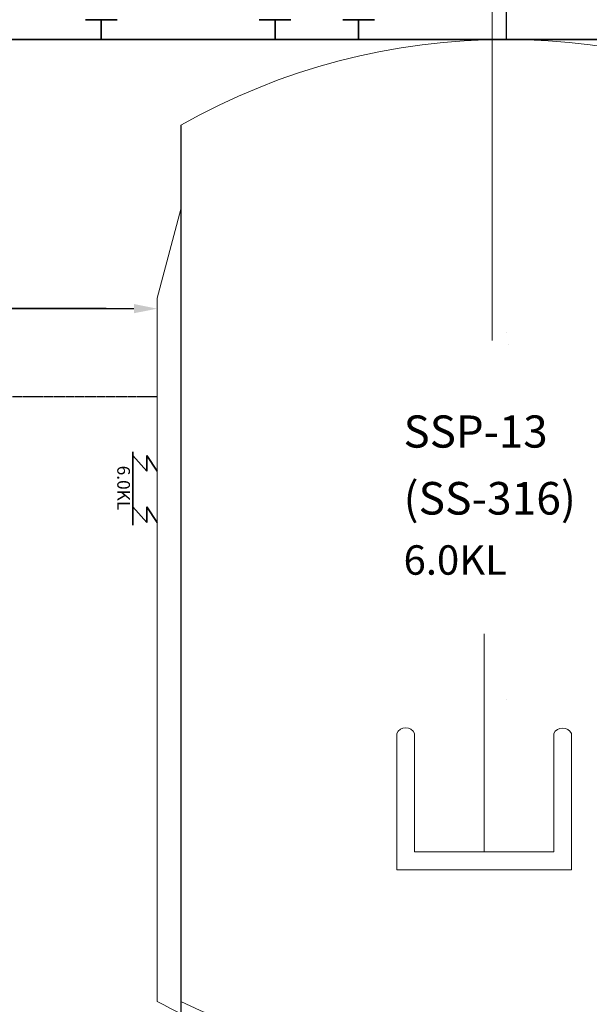
# Model space of a CAD drawing. Units: millimetres. Extents: x 353872 to 441597, y 126154 to 187356.
# Tile 8 of 28: x 390443 to 394852, y 141663 to 149281. Entities that reach past the tile are written whole.
import ezdxf

# ---------------------------------------------------------------- set-up
doc = ezdxf.new("R2010")
doc.units = ezdxf.units.MM
doc.linetypes.add('ACAD_ISO02W100', pattern=[15, 12, -3])
for name, color, linetype, lineweight in [('A-ANNO-DIMS', 2, 'Continuous', 18), ('P-ANNO-SYMB', 7, 'Continuous', 18), ('P-ANNO-TEXT', 7, 'Continuous', 25), ('P-BNDY', 4, 'ACAD_ISO02W100', 25), ('P-INST-SIGN', 4, 'Continuous', 18), ('P-PIPE', 3, 'Continuous', 35), ('P-PIPE-FITT', 6, 'Continuous', 25)]:
    doc.layers.add(name, color=color, linetype=linetype, lineweight=lineweight)
doc.layers.add('AC-UINT', color=2, linetype='Continuous')
doc.styles.get("Standard").update_dxf_attribs({"font": 'arial.ttf'})
doc.dimstyles.get("Standard").update_dxf_attribs({"dimtxt": 0.18, "dimasz": 0.18, "dimexe": 0.18, "dimexo": 0.0625, "dimgap": 0.09, "dimtad": 0, "dimtih": 1, "dimtoh": 1, "dimdec": 4, "dimzin": 0, "dimdsep": 46, "dimtxsty": 'Standard', "dimcen": 0.09, "dimadec": 0, "dimazin": 0, "dimtfac": 1, "dimtdec": 4, "dimtofl": 0, "dimtmove": 0, "dimatfit": 3, "dimfxl": 1, "dimtolj": 1, "dimtzin": 0, "dimarcsym": 0})

# ---------------------------------------------------------------- blocks, each defined once
blk = doc.blocks.new('DFSG')
at = {"layer": 'AC-UINT', "ltscale": 3}
blk.add_line((94.3237, -27.1601), (94.091, -27.1601), dxfattribs=at)
blk.add_solid([(94.091, -27.1214), (94.0909, -27.1989), (93.8965, -27.1598)], dxfattribs=at)
blk = doc.blocks.new('*D29')
at = {"layer": 'A-ANNO-DIMS', "color": 0, "lineweight": -2, "transparency": 16777216}
for p, q in [((391689.9, 148464.5), (391689.9, 133812.7)), ((396727.5, 148464.5), (396727.5, 133812.7)), ((391690.1, 133812.8), (394208.4, 133812.8)), ((396727.3, 133812.8), (394209.1, 133812.8))]:
    blk.add_line(p, q, dxfattribs=at)
at = {"layer": 'A-ANNO-DIMS', "color": 0, "transparency": 16777216}
for points in [[(391690.1, 133812.9), (391690.1, 133812.8), (391689.9, 133812.8)], [(396727.3, 133812.9), (396727.3, 133812.8), (396727.5, 133812.8)]]:
    blk.add_solid(points, dxfattribs=at)
at = {"layer": 'Defpoints', "color": 0, "transparency": 16777216}
for p in [(391689.9, 148464.5), (396727.5, 148464.5), (396727.5, 133812.8)]:
    blk.add_point(p, dxfattribs=at)
at = {"layer": 'A-ANNO-DIMS', "color": 0, "transparency": 16777216, "insert": (394208.7, 133812.8), "char_height": 0.18, "attachment_point": 5}
blk.add_mtext('\\A1;5038', dxfattribs=at)
blk = doc.blocks.new('*D35')
at = {"layer": 'A-ANNO-DIMS', "color": 0, "lineweight": -2, "transparency": 16777216}
for p, q in [((394208.5, 152192.2), (394208.7, 152192.2)), ((394208.7, 152192.2), (394208.7, 149129.3)), ((394208.6, 144024.1), (394208.8, 144024.1)), ((394208.7, 144024), (394208.7, 144024.2))]:
    blk.add_line(p, q, dxfattribs=at)
at = {"layer": 'A-ANNO-DIMS', "color": 0, "transparency": 16777216}
blk.add_solid([(394208.7, 149129.3), (394208.7, 149129.3), (394208.7, 149129.2)], dxfattribs=at)
at = {"layer": 'Defpoints', "color": 0, "transparency": 16777216}
for p in [(394208.7, 149129.2), (394208.7, 144024.1)]:
    blk.add_point(p, dxfattribs=at)
at = {"layer": 'A-ANNO-DIMS', "color": 0, "transparency": 16777216, "insert": (394208.1, 152192.2), "char_height": 0.18, "attachment_point": 5}
blk.add_mtext('\\A1;R5105', dxfattribs=at)
blk = doc.blocks.new('*D36')
at = {"layer": 'A-ANNO-DIMS', "color": 0, "lineweight": -2, "transparency": 16777216}
for p, q in [((394208.6, 146860.2), (394208.8, 146860.2)), ((394208.7, 146860.2), (394208.7, 146860.3)), ((394208.7, 137652.4), (394208.7, 141105.1)), ((394208.5, 137652.4), (394208.7, 137652.4))]:
    blk.add_line(p, q, dxfattribs=at)
at = {"layer": 'A-ANNO-DIMS', "color": 0, "transparency": 16777216}
blk.add_solid([(394208.7, 141105.1), (394208.7, 141105.1), (394208.7, 141105.3)], dxfattribs=at)
at = {"layer": 'Defpoints', "color": 0, "transparency": 16777216}
for p in [(394208.7, 146860.2), (394208.7, 141105.3)]:
    blk.add_point(p, dxfattribs=at)
at = {"layer": 'A-ANNO-DIMS', "color": 0, "transparency": 16777216, "insert": (394208.1, 137652.4), "char_height": 0.18, "attachment_point": 5}
blk.add_mtext('\\A1;R5755', dxfattribs=at)
blk = doc.blocks.new('*D37')
at = {"layer": 'A-ANNO-DIMS', "color": 0, "lineweight": -2, "transparency": 16777216}
for p, q in [((394230.3, 146766.2), (394230.5, 146766.2)), ((394230.4, 146766.1), (394230.4, 146766.3)), ((391240.8, 138041.4), (392361.8, 141313)), ((391240.6, 138041.4), (391240.8, 138041.4))]:
    blk.add_line(p, q, dxfattribs=at)
at = {"layer": 'A-ANNO-DIMS', "color": 0, "transparency": 16777216}
blk.add_solid([(392361.8, 141313), (392361.9, 141313), (392361.9, 141313.2)], dxfattribs=at)
at = {"layer": 'Defpoints', "color": 0, "transparency": 16777216}
for p in [(394230.4, 146766.2), (392361.9, 141313.2)]:
    blk.add_point(p, dxfattribs=at)
at = {"layer": 'A-ANNO-DIMS', "color": 0, "transparency": 16777216, "insert": (391240, 138041.4), "char_height": 0.18, "attachment_point": 5}
blk.add_mtext('\\A1;2X R5764', dxfattribs=at)

msp = doc.modelspace()

# ---------------------------------------------------------------- linework, layer by layer
at = {"layer": 'P-ANNO-SYMB'}
for p, q in [((394099.49, 149129.17), (394099.49, 146800.09)), ((394038.38, 142843.34), (394038.38, 144530.58))]:
    msp.add_line(p, q, dxfattribs=at)
at = {"layer": 'P-BNDY'}
msp.add_line((360736.55, 146365.61), (391507.08, 146365.61), dxfattribs=at)
at = {"layer": 'P-INST-SIGN'}
for p, q in [((394099.49, 149129.17), (394099.49, 149343.39)), ((394208.72, 149129.17), (394208.72, 149343.39)), ((391507.08, 147126.17), (391689.9, 147816.11))]:
    msp.add_line(p, q, dxfattribs=at)
for points in [[(391689.9, 141685.82), (391689.9, 148464.52)], [(391507.08, 141685.82), (391507.08, 147126.17)], [(393361.4, 143759.11), (393361.4, 142704.59), (394715.35, 142704.59), (394715.35, 143759.11)], [(393500.15, 143759.11), (393500.15, 142843.34), (394576.6, 142843.34), (394576.6, 143759.11)]]:
    msp.add_lwpolyline(points, dxfattribs=at)
for centre, radius, start, end in [((394208.72, 144024.11), 5105.06, 60.436001, 119.563999), ((393430.78, 143724.9), 77.35, 26.242849, 153.757151), ((394645.98, 143719.49), 79.89, 29.726445, 150.273555), ((394230.39, 146766.22), 5764.27, 241.806793, 260.3645), ((394208.72, 146860.25), 5754.92, 244.04409, 295.95591)]:
    msp.add_arc(centre, radius, start, end, dxfattribs=at)
at = {"layer": 'P-PIPE'}
for p, q in [((391196.72, 149280.57), (390951.96, 149280.57)), ((391074.34, 149280.57), (391074.34, 149129.17)), ((392542.13, 149280.57), (392297.37, 149280.57)), ((392419.75, 149280.57), (392419.75, 149129.17)), ((393189.09, 149280.57), (392944.33, 149280.57)), ((393066.71, 149280.57), (393066.71, 149129.17)), ((386450.69, 149129.17), (407087.67, 149129.17)), ((388692.41, 147045.54), (391112.65, 147045.74)), ((391318.56, 145936.47), (391318.56, 145371.03)), ((391426.99, 145787.97), (391318.56, 145909.82)), ((391507.08, 145787.97), (391426.99, 145909.82)), ((391426.99, 145909.82), (391426.99, 145787.97)), ((391426.99, 145391.48), (391318.56, 145513.33)), ((391507.08, 145391.48), (391426.99, 145513.33)), ((391426.99, 145513.33), (391426.99, 145391.48))]:
    msp.add_line(p, q, dxfattribs=at)

# ---------------------------------------------------------------- block references
at = {"layer": 'P-PIPE-FITT', "xscale": 923.3484342094463, "yscale": 923.3484342094463, "zscale": 923.3484342094463, "rotation": 179.9589088552121}
msp.add_blockref('DFSG', (478188.28, 121905.03), dxfattribs=at)

# ---------------------------------------------------------------- texts
at = {"layer": 'P-ANNO-TEXT'}
for s, height, p in [('SSP-13', 249.092, (393414.61, 145970.22)), ('(SS-316)', 252.078, (393414.61, 145452.13)), ('6.0KL', 227.502, (393414.61, 144986.9))]:
    msp.add_text(s, height=height, dxfattribs=at).set_placement(p)
msp.add_text('6.0KL', height=98.09, rotation=270, dxfattribs=at).set_placement((391198.6, 145830.62))

# ---------------------------------------------------------------- dimensions: what is measured, and where the dimension line sits
at = {"layer": 'A-ANNO-DIMS'}
for center, mpoint, picture, middle in [((394208.72, 144024.11), (394208.7, 149129.17), '*D35', (394208.07, 152192.2)), ((394208.72, 146860.25), (394208.7, 141105.33), '*D36', (394208.07, 137652.37))]:
    dim = msp.add_radius_dim(center=center, mpoint=mpoint, dimstyle='Standard', override={"dimdec": 0, "dimlfac": 1, "dimrnd": 0, "dimzin": 0, "dimdsep": 46, "dimlunit": 2}, dxfattribs=at)
    dim.commit()
    dim.dimension.update_dxf_attribs({"geometry": picture, "text_midpoint": middle, "dimtype": 164})
dim = msp.add_linear_dim(base=(396727.53, 133812.84), p1=(391689.9, 148464.52), p2=(396727.53, 148464.52), dimstyle='Standard', override={"dimdec": 0, "dimlfac": 1, "dimrnd": 0, "dimzin": 0, "dimdsep": 46, "dimlunit": 2}, dxfattribs=at)
dim.commit()
dim.dimension.update_dxf_attribs({"geometry": '*D29', "text_midpoint": (394208.72, 133812.84)})
dim = msp.add_radius_dim(center=(394230.39, 146766.22), mpoint=(392361.89, 141313.18), text='2X <>', dimstyle='Standard', override={"dimdec": 0, "dimlfac": 1, "dimrnd": 0, "dimzin": 0, "dimdsep": 46, "dimlunit": 2}, dxfattribs=at)
dim.commit()
dim.dimension.update_dxf_attribs({"geometry": '*D37', "text_midpoint": (391239.98, 138041.36), "dimtype": 164})

doc.saveas('drawing.dxf')
